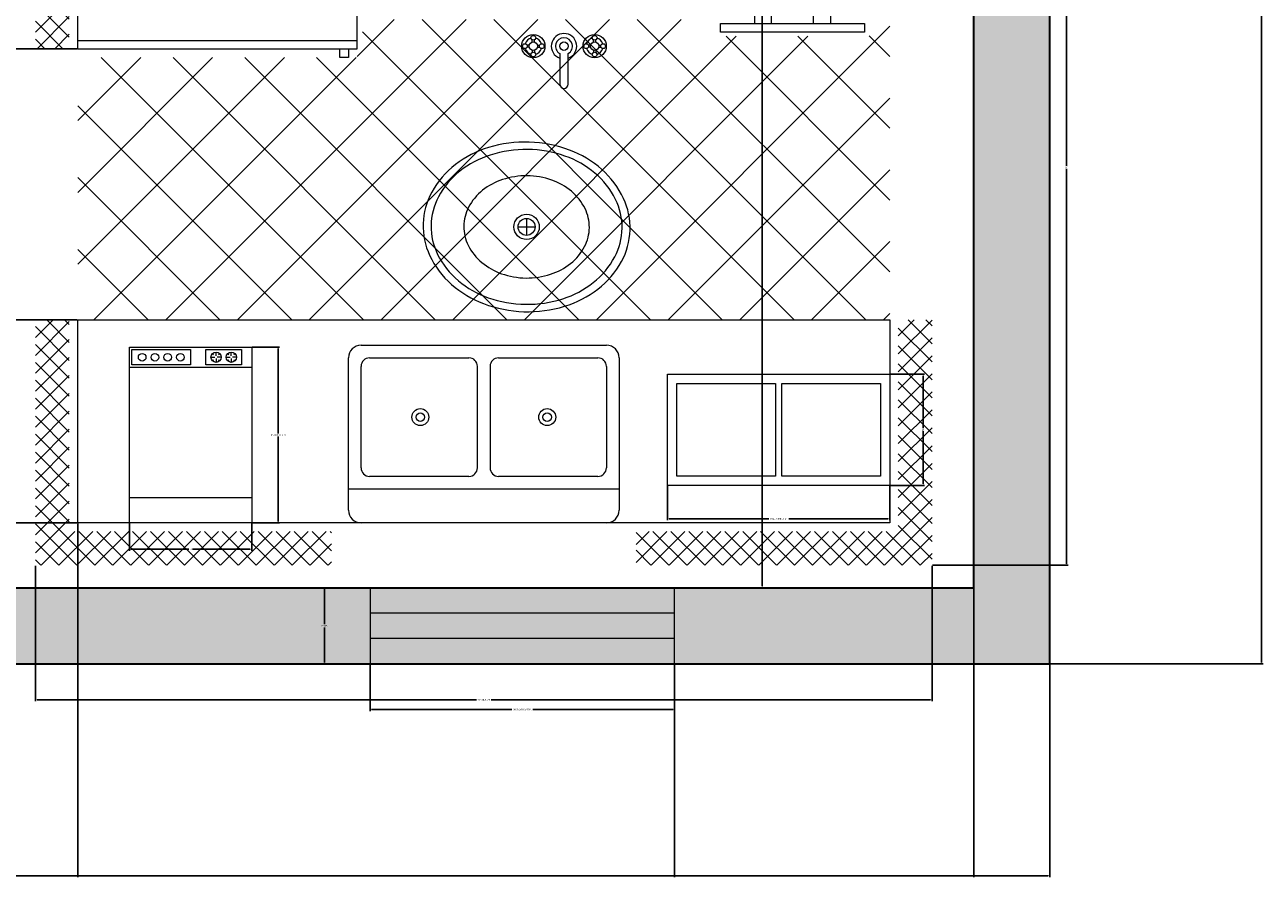
# Model space of a CAD drawing. Units: inches. Extents: x 1434 to 1845, y 1483 to 2014.
# Tile 6 of 11: x 1698 to 1845, y 1483 to 1584. Entities that reach past the tile are written whole.
import ezdxf

# ---------------------------------------------------------------- set-up
doc = ezdxf.new("R2010")
doc.units = ezdxf.units.IN
for name, color, linetype, lineweight in [('A-ANNO-DIMS', 2, 'Continuous', 18), ('A-EQPM', 9, 'Continuous', 18), ('A-FLOR-CASE', 8, 'Continuous', 18), ('A-FLOR-FIXT', 8, 'Continuous', 18), ('A-GLAZ', 4, 'Continuous', 18), ('A-GLAZ-PATT', 9, 'Continuous', 13), ('A-WALL', 7, 'Continuous', 35), ('A-WALL-PATT', 8, 'Continuous', 13)]:
    doc.layers.add(name, color=color, linetype=linetype, lineweight=lineweight)
doc.styles.get("Standard").update_dxf_attribs({"font": 'arial.ttf'})
doc.dimstyles.get("Standard").update_dxf_attribs({"dimtxt": 0.18, "dimasz": 0.18, "dimexe": 0.18, "dimexo": 0.0625, "dimgap": 0.09, "dimtad": 0, "dimtih": 1, "dimtoh": 1, "dimdec": 4, "dimzin": 0, "dimdsep": 46, "dimtxsty": 'Standard', "dimcen": 0.09, "dimadec": 0, "dimazin": 0, "dimtfac": 1, "dimtdec": 4, "dimtofl": 0, "dimtmove": 0, "dimatfit": 3, "dimfxl": 1, "dimtolj": 1, "dimtzin": 0, "dimarcsym": 0})

# ---------------------------------------------------------------- blocks, each defined once
blk = doc.blocks.new('Sink - Oval top')
for p, q in [((-1, 0), (1, 0)), ((0, 1), (0, -1))]:
    blk.add_line(p, q)
for points in [[(-12.23, 0.39, 0.117634), (-11.46, -3.36, 0.104469), (-8.88, -6.8, 0.090016), (-5.08, -9.07, 0.08192), (-0.32, -10.02, 0.08192), (4.49, -9.38, 0.090016), (8.42, -7.36, 0.104469), (11.22, -4.09, 0.117634), (12.23, -0.39, 0.117634), (11.46, 3.36, 0.104469), (8.88, 6.8, 0.090016), (5.08, 9.07, 0.08192), (0.32, 10.02, 0.08192), (-4.49, 9.38, 0.090016), (-8.42, 7.36, 0.104469), (-11.22, 4.09, 0.117634)], [(-11.29, 0.16, 0.118622), (-10.52, -3.25, 0.104678), (-8.07, -6.36, 0.089562), (-4.54, -8.37, 0.081185), (-0.13, -9.15, 0.081185), (4.3, -8.49, 0.089562), (7.89, -6.58, 0.104678), (10.42, -3.55, 0.118622), (11.29, -0.16, 0.118622), (10.52, 3.25, 0.104678), (8.07, 6.36, 0.089562), (4.54, 8.37, 0.081185), (0.13, 9.15, 0.081185), (-4.3, 8.49, 0.089562), (-7.89, 6.58, 0.104678), (-10.42, 3.55, 0.118622)], [(-7.42, 0.08, 0.118283), (-6.91, -2.17, 0.104607), (-5.29, -4.21, 0.089718), (-2.97, -5.53, 0.081436), (-0.07, -6.04, 0.081436), (2.84, -5.59, 0.089718), (5.2, -4.33, 0.104607), (6.86, -2.32, 0.118283), (7.42, -0.08, 0.118283), (6.91, 2.17, 0.104607), (5.29, 4.21, 0.089718), (2.97, 5.53, 0.081436), (0.07, 6.04, 0.081436), (-2.84, 5.59, 0.089718), (-5.2, 4.33, 0.104607), (-6.86, 2.32, 0.118283)]]:
    blk.add_lwpolyline(points, format="xyb", close=True)
for radius in [1.5, 1]:
    blk.add_circle((0, 0), radius)
blk = doc.blocks.new('Faucet - Bathroom top')
for p, q in [((-4.107, 0.125), (-4.375, 0.125)), ((-3.75, 0.4788), (-3.75, 0.75)), ((-3.5, 0.482), (-3.5, 0.75)), ((-3.1461, 0.125), (-2.875, 0.125)), ((3.143, 0.125), (2.875, 0.125)), ((3.5, 0.4788), (3.5, 0.75)), ((3.75, 0.482), (3.75, 0.75)), ((4.1039, 0.125), (4.375, 0.125)), ((-4.1039, -0.125), (-4.375, -0.125)), ((-3.75, -0.4821), (-3.75, -0.75)), ((-3.5, -0.4789), (-3.5, -0.75)), ((-3.143, -0.125), (-2.875, -0.125)), ((-0.5, -0.8639), (-0.5, -4.5)), ((0.5, -4.5), (0.5, -0.8631)), ((3.1461, -0.125), (2.875, -0.125)), ((3.5, -0.4821), (3.5, -0.75)), ((3.75, -0.4789), (3.75, -0.75)), ((4.107, -0.125), (4.375, -0.125))]:
    blk.add_line(p, q)
for centre, radius in [((-3.625, 0), 1.375), ((-4.625, 0), 0.2795), ((-3.625, 0), 0.5), ((-3.625, 1), 0.2795), ((-2.625, 0), 0.2795), ((0, 0), 0.5), ((3.625, 0), 1.375), ((2.625, 0), 0.2795), ((3.625, 0), 0.5), ((3.625, 1), 0.2795), ((4.625, 0), 0.2795), ((-3.625, -1), 0.2795), ((3.625, -1), 0.2795)]:
    blk.add_circle(centre, radius)
for centre, radius, start, end in [((0, 0), 1.5, 289.6514, 250.3603), ((-3.625, 0), 1, 105.2407, 164.2093), ((-3.625, 0), 1, 16.44125, 74.07887), ((0, 0), 1, 300.3431, 239.7554), ((3.625, 0), 1, 106.12, 164.0884), ((3.625, 0), 1, 16.23422, 73.90469), ((-3.625, 0), 1, 196.2342, 253.9047), ((-3.625, 0), 1, 286.12, 344.0884), ((3.625, 0), 1, 196.4413, 254.0789), ((3.625, 0), 1, 285.2407, 344.2093), ((0, -4.5), 0.5, 180, 0)]:
    blk.add_arc(centre, radius, start, end)
blk = doc.blocks.new('Kitchen Layout - 7 x 8 ft')
for p, q in [((-5, 81.32), (2.68, 89)), ((-5, 83.44), (0.56, 89)), ((-5, 85.56), (-1.56, 89)), ((-5, 87.68), (-3.68, 89)), ((-1, 84.97), (-5, 88.97)), ((1.09, 85), (-2.91, 89)), ((3.21, 85), (-0.79, 89)), ((0.81, 85), (4.81, 89)), ((5.34, 85), (1.34, 89)), ((2.93, 85), (6.93, 89)), ((7.46, 85), (3.46, 89)), ((5.05, 85), (9.05, 89)), ((9.58, 85), (5.58, 89)), ((7.17, 85), (11.17, 89)), ((11.7, 85), (7.7, 89)), ((9.29, 85), (13.29, 89)), ((13.82, 85), (9.82, 89)), ((11.41, 85), (15.41, 89)), ((15.94, 85), (11.94, 89)), ((13.53, 85), (17.53, 89)), ((18.06, 85), (14.06, 89)), ((15.65, 85), (19.65, 89)), ((20.18, 85), (16.18, 89)), ((17.78, 85), (21.78, 89)), ((22.31, 85), (18.31, 89)), ((19.9, 85), (23.9, 89)), ((24.43, 85), (20.43, 89)), ((22.02, 85), (26.02, 89)), ((26.55, 85), (22.55, 89)), ((24.14, 85), (28.14, 89)), ((28.67, 85), (24.67, 89)), ((26.26, 85), (30.26, 89)), ((30.79, 85), (26.79, 89)), ((28.38, 85), (32.38, 89)), ((32.91, 85), (28.91, 89)), ((30.5, 85), (34.5, 89)), ((35.03, 85), (31.03, 89)), ((32.63, 85), (36.63, 89)), ((37.16, 85), (33.16, 89)), ((34.75, 85), (38.75, 89)), ((39.28, 85), (35.28, 89)), ((36.87, 85), (40.87, 89)), ((41.4, 85), (37.4, 89)), ((38.99, 85), (42.99, 89)), ((43.52, 85), (39.52, 89)), ((41.11, 85), (45.11, 89)), ((45.64, 85), (41.64, 89)), ((43.23, 85), (47.23, 89)), ((47.76, 85), (43.76, 89)), ((45.35, 85), (49.35, 89)), ((49.88, 85), (45.88, 89)), ((47.47, 85), (51.47, 89)), ((52, 85), (48, 89)), ((49.6, 85), (53.6, 89)), ((54.13, 85), (50.13, 89)), ((51.72, 85), (55.72, 89)), ((56.25, 85), (52.25, 89)), ((53.84, 85), (57.84, 89)), ((58.37, 85), (54.37, 89)), ((55.96, 85), (59.96, 89)), ((60.49, 85), (56.49, 89)), ((58.08, 85), (62.08, 89)), ((62.61, 85), (58.61, 89)), ((60.2, 85), (64.2, 89)), ((64.73, 85), (60.73, 89)), ((62.32, 85), (66.32, 89)), ((66.85, 85), (62.85, 89)), ((64.45, 85), (68.45, 89)), ((68.97, 85), (64.97, 89)), ((66.57, 85), (70.57, 89)), ((71.1, 85), (67.1, 89)), ((68.69, 85), (72.69, 89)), ((73.22, 85), (69.22, 89)), ((70.81, 85), (74.81, 89)), ((75.34, 85), (71.34, 89)), ((72.93, 85), (76.93, 89)), ((77.46, 85), (73.46, 89)), ((75.05, 85), (79.05, 89)), ((79.58, 85), (75.58, 89)), ((77.17, 85), (81.17, 89)), ((81.7, 85), (77.7, 89)), ((79.29, 85), (83.29, 89)), ((83.82, 85), (79.82, 89)), ((81.42, 85), (85.42, 89)), ((85.95, 85), (81.95, 89)), ((83.54, 85), (87.54, 89)), ((88.07, 85), (84.07, 89)), ((85.66, 85), (89.66, 89)), ((90.19, 85), (86.19, 89)), ((87.78, 85), (91.78, 89)), ((92.31, 85), (88.31, 89)), ((89.9, 85), (93.9, 89)), ((94.43, 85), (90.43, 89)), ((92.02, 85), (96.02, 89)), ((96.55, 85), (92.55, 89)), ((94.14, 85), (98.14, 89)), ((101, 82.67), (94.67, 89)), ((96.27, 85), (100.27, 89)), ((101, 84.79), (96.79, 89)), ((101, 86.92), (98.92, 89)), ((-1, 82.85), (-5, 86.85)), ((97, 83.61), (101, 87.61)), ((97, 81.49), (101, 85.49)), ((-1, 80.73), (-5, 84.73)), ((34, 84), (96, 84)), ((34, 60), (34, 84)), ((96, 84), (96, 60)), ((101, 80.55), (97, 84.55)), ((-5, 79.19), (-1, 83.19)), ((-1, 78.61), (-5, 82.61)), ((97, 79.37), (101, 83.37)), ((101, 78.43), (97, 82.43)), ((-5, 77.07), (-1, 81.07)), ((74, 81), (95, 81)), ((97, 77.25), (101, 81.25)), ((-1, 76.49), (-5, 80.49)), ((101, 76.31), (97, 80.31)), ((97, 75.13), (101, 79.13)), ((-5, 74.95), (-1, 78.95)), ((-1, 74.36), (-5, 78.36)), ((101, 74.19), (97, 78.19)), ((-5, 72.83), (-1, 76.83)), ((-1, 72.24), (-5, 76.24)), ((97, 73.01), (101, 77.01)), ((-5, 70.71), (-1, 74.71)), ((101, 72.07), (97, 76.07)), ((97, 70.89), (101, 74.89)), ((-1, 70.12), (-5, 74.12)), ((101, 69.95), (97, 73.95)), ((-5, 68.59), (-1, 72.59)), ((-1, 68), (-5, 72)), ((97, 68.76), (101, 72.76)), ((101, 67.82), (97, 71.82)), ((-5, 66.47), (-1, 70.47)), ((97, 66.64), (101, 70.64)), ((-1, 65.88), (-5, 69.88)), ((101, 65.7), (97, 69.7)), ((-5, 64.35), (-1, 68.35)), ((-1, 63.76), (-5, 67.76)), ((97, 64.52), (101, 68.52)), ((101, 63.58), (97, 67.58)), ((-5, 62.22), (-1, 66.22)), ((97, 62.4), (101, 66.4)), ((-1, 61.64), (-5, 65.64)), ((101, 61.46), (97, 65.46)), ((-5, 60.1), (-1, 64.1)), ((-1, 59.52), (-5, 63.52)), ((97, 60.28), (101, 64.28)), ((100.34, 60), (97, 63.34)), ((-5, 57.98), (-1, 61.98)), ((98.84, 60), (101, 62.16)), ((-1, 57.39), (-5, 61.39)), ((98.22, 60), (97, 61.22)), ((100.96, 60), (101, 60.04)), ((-1.73, 56), (-5, 59.27)), ((-4.86, 56), (-1, 59.86)), ((10.4, 24), (45.9, 59.5)), ((18.88, 24), (54.38, 59.5)), ((27.37, 24), (62.87, 59.5)), ((33.03, 55.11), (37.41, 59.5)), ((96, 60), (34, 60)), ((35.85, 24), (71.35, 59.5)), ((76.2, 24), (40.7, 59.5)), ((84.68, 24), (49.18, 59.5)), ((93.17, 24), (57.67, 59.5)), ((61.31, 24), (96, 58.69)), ((96, 29.65), (66.15, 59.5)), ((80, 60), (80, 59)), ((82, 59), (82, 60)), ((87, 59), (87, 60)), ((89, 60), (89, 59)), ((-3.85, 56), (-5, 57.15)), ((-2.74, 56), (-1, 57.74)), ((67.71, 24), (33.68, 58.04)), ((44.34, 24), (77.84, 57.5)), ((52.82, 24), (86.32, 57.5)), ((96, 38.14), (76.64, 57.5)), ((96, 46.63), (85.13, 57.5)), ((96, 55.11), (93.57, 57.54)), ((0, 57), (33, 57)), ((31, 55), (31, 56)), ((32, 56), (32, 55)), ((0, 30.57), (24.43, 55)), ((0, 39.06), (15.94, 55)), ((0, 47.54), (7.46, 55)), ((1.91, 24), (32.91, 55)), ((33.77, 24), (2.77, 55)), ((42.26, 24), (11.26, 55)), ((50.74, 24), (19.74, 55)), ((59.23, 24), (28.23, 55)), ((32, 55), (31, 55)), ((69.79, 24), (96, 50.21)), ((25.29, 24), (0, 49.29)), ((78.28, 24), (96, 41.72)), ((16.8, 24), (0, 40.8)), ((8.32, 24), (0, 32.32)), ((86.76, 24), (96, 33.24)), ((-5, 21.92), (-2.92, 24)), ((-5, 19.8), (-1, 23.8)), ((-1, 21.33), (-3.67, 24)), ((-1, 23.45), (-1.55, 24)), ((0, 24), (96, 24)), ((0, 0), (0, 24)), ((95.25, 24), (96, 24.75)), ((96, 24), (96, 0)), ((97, 22.1), (98.9, 24)), ((97, 19.97), (101, 23.97)), ((101, 21.16), (98.16, 24)), ((101, 23.28), (100.28, 24)), ((-1, 19.21), (-5, 23.21)), ((101, 19.03), (97, 23.03)), ((-5, 17.68), (-1, 21.68)), ((-1, 17.09), (-5, 21.09)), ((97, 17.85), (101, 21.85)), ((101, 16.91), (97, 20.91)), ((-5, 15.55), (-1, 19.55)), ((97, 15.73), (101, 19.73)), ((-1, 14.97), (-5, 18.97)), ((47.25, 6.5), (47.25, 18.5)), ((48.75, 18.5), (48.75, 6.5)), ((101, 14.79), (97, 18.79)), ((97, 13.61), (101, 17.61)), ((-5, 13.43), (-1, 17.43)), ((-1, 12.85), (-5, 16.85)), ((101, 12.67), (97, 16.67)), ((-5, 11.31), (-1, 15.31)), ((-1, 10.73), (-5, 14.73)), ((97, 11.49), (101, 15.49)), ((-5, 9.19), (-1, 13.19)), ((101, 10.55), (97, 14.55)), ((97, 9.37), (101, 13.37)), ((-1, 8.6), (-5, 12.6)), ((101, 8.43), (97, 12.43)), ((-5, 7.07), (-1, 11.07)), ((-1, 6.48), (-5, 10.48)), ((97, 7.25), (101, 11.25)), ((101, 6.31), (97, 10.31)), ((-5, 4.95), (-1, 8.95)), ((97, 5.12), (101, 9.12)), ((-1, 4.36), (-5, 8.36)), ((101, 4.18), (97, 8.18)), ((-5, 2.83), (-1, 6.83)), ((-1, 2.24), (-5, 6.24)), ((97, 3), (101, 7)), ((101, 2.06), (97, 6.06)), ((-5, 0.71), (-1, 4.71)), ((97, 0.88), (101, 4.88)), ((-1, 0.12), (-5, 4.12)), ((64, 4), (32, 4)), ((101, -0.06), (97, 3.94)), ((-5, -1.42), (-1, 2.58)), ((2, -5), (-5, 2)), ((93.24, -5), (101, 2.76)), ((101, -2.18), (97, 1.82)), ((-5, -3.54), (-1, 0.46)), ((96, 0), (0, 0)), ((95.36, -5), (101, 0.64)), ((-0.12, -5), (-5, -0.12)), ((-4.34, -5), (-0.34, -1)), ((-2.22, -5), (1.78, -1)), ((-0.1, -5), (3.9, -1)), ((4.12, -5), (0.12, -1)), ((2.02, -5), (6.02, -1)), ((6.24, -5), (2.24, -1)), ((4.14, -5), (8.14, -1)), ((8.36, -5), (4.36, -1)), ((6.27, -5), (10.27, -1)), ((10.48, -5), (6.48, -1)), ((8.39, -5), (12.39, -1)), ((12.6, -5), (8.6, -1)), ((10.51, -5), (14.51, -1)), ((14.73, -5), (10.73, -1)), ((12.63, -5), (16.63, -1)), ((16.85, -5), (12.85, -1)), ((14.75, -5), (18.75, -1)), ((18.97, -5), (14.97, -1)), ((16.87, -5), (20.87, -1)), ((21.09, -5), (17.09, -1)), ((18.99, -5), (22.99, -1)), ((23.21, -5), (19.21, -1)), ((21.11, -5), (25.11, -1)), ((25.33, -5), (21.33, -1)), ((23.24, -5), (27.24, -1)), ((27.45, -5), (23.45, -1)), ((25.36, -5), (29.36, -1)), ((29.57, -5), (25.57, -1)), ((30, -3.3), (27.7, -1)), ((30, -1.18), (29.82, -1)), ((66, -2.54), (67.54, -1)), ((66, -4.66), (69.66, -1)), ((69.88, -5), (66, -1.12)), ((67.78, -5), (71.78, -1)), ((72, -5), (68, -1)), ((69.9, -5), (73.9, -1)), ((74.12, -5), (70.12, -1)), ((72.03, -5), (76.03, -1)), ((76.24, -5), (72.24, -1)), ((74.15, -5), (78.15, -1)), ((78.36, -5), (74.36, -1)), ((76.27, -5), (80.27, -1)), ((80.49, -5), (76.49, -1)), ((78.39, -5), (82.39, -1)), ((82.61, -5), (78.61, -1)), ((80.51, -5), (84.51, -1)), ((84.73, -5), (80.73, -1)), ((82.63, -5), (86.63, -1)), ((86.85, -5), (82.85, -1)), ((84.75, -5), (88.75, -1)), ((88.97, -5), (84.97, -1)), ((86.88, -5), (90.88, -1)), ((91.09, -5), (87.09, -1)), ((89, -5), (93, -1)), ((93.21, -5), (89.21, -1)), ((91.12, -5), (95.12, -1)), ((95.34, -5), (91.34, -1)), ((97.46, -5), (93.46, -1)), ((99.58, -5), (95.58, -1)), ((101, -4.3), (97, -0.3)), ((-2.25, -5), (-5, -2.25)), ((27.48, -5), (30, -2.48)), ((97.48, -5), (101, -1.48)), ((-4.37, -5), (-5, -4.37)), ((67.76, -5), (66, -3.24)), ((99.6, -5), (101, -3.6)), ((29.6, -5), (30, -4.6))]:
    blk.add_line(p, q)
for points in [[(0, 56), (0, 84), (33, 84), (33, 56)], [(74, 60), (74, 84), (95, 84), (95, 60)], [(76, 58), (76, 59), (93, 59), (93, 58)]]:
    blk.add_lwpolyline(points, close=True)
for points in [[(33.5, 21), (62.5, 21)], [(32, 1.5), (32, 19.5)], [(34.5, 19.5), (46.25, 19.5)], [(49.75, 19.5), (61.5, 19.5)], [(64, 19.5), (64, 1.5)], [(33.5, 6.5), (33.5, 18.5)], [(62.5, 18.5), (62.5, 6.5)], [(46.25, 5.5), (34.5, 5.5)], [(61.5, 5.5), (49.75, 5.5)], [(62.5, 0), (33.5, 0)]]:
    blk.add_lwpolyline(points)
for centre, radius in [((80, 75), 4), ((80, 75), 3), ((89, 75), 3), ((80, 75), 2), ((89, 75), 2), ((80, 75), 1), ((89, 75), 1), ((80, 66), 3), ((89, 66), 4), ((89, 66), 3), ((80, 66), 2), ((89, 66), 2), ((80, 66), 1), ((89, 66), 1), ((40.5, 12.5), 1), ((55.5, 12.5), 1), ((40.5, 12.5), 0.5), ((55.5, 12.5), 0.5)]:
    blk.add_circle(centre, radius)
for centre, radius, start, end in [((33.5, 19.5), 1.5, 90, 180), ((62.5, 19.5), 1.5, 0, 90), ((34.5, 18.5), 1, 90, 180), ((46.25, 18.5), 1, 0, 90), ((49.75, 18.5), 1, 90, 180), ((61.5, 18.5), 1, 0, 90), ((34.5, 6.5), 1, 180, 270), ((46.25, 6.5), 1, 270, 0), ((49.75, 6.5), 1, 180, 270), ((61.5, 6.5), 1, 270, 0), ((33.5, 1.5), 1.5, 180, 270), ((62.5, 1.5), 1.5, 270, 0)]:
    blk.add_arc(centre, radius, start, end)
blk = doc.blocks.new('Dishwasher')
for p, q in [((16, 32.5), (16.75, 32.5)), ((16.5, 32), (16.2942, 31.7942)), ((16.3156, 33.1843), (16.5, 33)), ((17, 32.75), (17, 33.5)), ((17, 32.25), (17, 31.5)), ((18, 32.5), (17.25, 32.5)), ((17.5, 33), (17.6938, 33.1938)), ((17.7061, 31.7939), (17.5, 32)), ((19, 32.5), (19.75, 32.5)), ((19.5, 32), (19.2942, 31.7942)), ((19.3156, 33.1843), (19.5, 33)), ((20, 32.75), (20, 33.5)), ((20, 32.25), (20, 31.5)), ((21, 32.5), (20.25, 32.5)), ((20.5, 33), (20.6938, 33.1938)), ((20.7061, 31.7939), (20.5, 32)), ((24, 30.5), (0, 30.5)), ((0, 5), (24, 5))]:
    blk.add_line(p, q)
for points in [[(0, 0), (0, 34.5), (24, 34.5), (24, 0)], [(0.5, 31), (0.5, 34), (12, 34), (12, 31)], [(15, 31), (15, 34), (22, 34), (22, 31)]]:
    blk.add_lwpolyline(points, close=True)
for centre, radius in [((2.5, 32.5), 0.75), ((5, 32.5), 0.75), ((7.5, 32.5), 0.75), ((10, 32.5), 0.75), ((17, 32.5), 1), ((20, 32.5), 1)]:
    blk.add_circle(centre, radius)
blk = doc.blocks.new('Wall Cabinet - 18 x 36 in front')
for p, q in [((17.5, -1.5), (17.5, -16.5)), ((18.5, -16.5), (18.5, -1.5))]:
    blk.add_line(p, q)
blk.add_lwpolyline([(0, -18), (0, 0), (36, 0), (36, -18)], close=True)
for points in [[(17.5, -16.5), (1.5, -16.5), (1.5, -1.5), (17.5, -1.5)], [(18.5, -1.5), (34.5, -1.5), (34.5, -16.5), (18.5, -16.5)]]:
    blk.add_lwpolyline(points)
blk = doc.blocks.new('WIN-36IN-9IN')
for p, q in [((3, 36), (3, 0)), ((6, 36), (6, 0))]:
    blk.add_line(p, q)
blk.add_lwpolyline([(9, 0), (9, 36), (0, 36), (0, 0)], close=True)
blk = doc.blocks.new('*D28')
at = {"layer": 'A-ANNO-DIMS', "color": 0, "lineweight": -2, "transparency": 16777216}
for p, q in [((1739.11, 1508.29), (1739.11, 1502.78)), ((1775.11, 1508.29), (1775.11, 1502.78)), ((1739.29, 1502.96), (1755.88, 1502.96)), ((1774.93, 1502.96), (1758.35, 1502.96))]:
    blk.add_line(p, q, dxfattribs=at)
at = {"layer": 'A-ANNO-DIMS', "color": 0, "transparency": 16777216}
for points in [[(1739.29, 1502.99), (1739.29, 1502.93), (1739.11, 1502.96)], [(1774.93, 1502.99), (1774.93, 1502.93), (1775.11, 1502.96)]]:
    blk.add_solid(points, dxfattribs=at)
at = {"layer": 'Defpoints', "color": 0, "transparency": 16777216}
for p in [(1739.11, 1508.36), (1775.11, 1508.36), (1775.11, 1502.96)]:
    blk.add_point(p, dxfattribs=at)
at = {"layer": 'A-ANNO-DIMS', "color": 0, "transparency": 16777216, "insert": (1757.11, 1502.96), "char_height": 0.18, "attachment_point": 5}
blk.add_mtext('\\A1;WINDOW B 36 TYP.', dxfattribs=at)
blk = doc.blocks.new('*D29')
at = {"layer": 'A-ANNO-DIMS', "color": 0, "lineweight": -2, "transparency": 16777216}
for p, q in [((1739.05, 1517.36), (1733.53, 1517.36)), ((1733.71, 1517.18), (1733.71, 1513.04)), ((1733.71, 1508.54), (1733.71, 1512.67)), ((1739.05, 1508.36), (1733.53, 1508.36))]:
    blk.add_line(p, q, dxfattribs=at)
at = {"layer": 'A-ANNO-DIMS', "color": 0, "transparency": 16777216}
for points in [[(1733.68, 1517.18), (1733.74, 1517.18), (1733.71, 1517.36)], [(1733.68, 1508.54), (1733.74, 1508.54), (1733.71, 1508.36)]]:
    blk.add_solid(points, dxfattribs=at)
at = {"layer": 'Defpoints', "color": 0, "transparency": 16777216}
for p in [(1739.11, 1517.36), (1733.71, 1508.36), (1739.11, 1508.36)]:
    blk.add_point(p, dxfattribs=at)
at = {"layer": 'A-ANNO-DIMS', "color": 0, "transparency": 16777216, "insert": (1733.71, 1512.86), "char_height": 0.18, "attachment_point": 5}
blk.add_mtext('\\A1;9 TYP.', dxfattribs=at)
blk = doc.blocks.new('*D46')
at = {"layer": 'A-ANNO-DIMS', "color": 0, "lineweight": -2, "transparency": 16777216}
for p, q in [((1699.55, 1519.96), (1699.55, 1503.94)), ((1805.55, 1519.96), (1805.55, 1503.94)), ((1699.73, 1504.12), (1751.68, 1504.12)), ((1805.37, 1504.12), (1753.42, 1504.12))]:
    blk.add_line(p, q, dxfattribs=at)
at = {"layer": 'A-ANNO-DIMS', "color": 0, "transparency": 16777216}
for points in [[(1699.73, 1504.15), (1699.73, 1504.09), (1699.55, 1504.12)], [(1805.37, 1504.15), (1805.37, 1504.09), (1805.55, 1504.12)]]:
    blk.add_solid(points, dxfattribs=at)
at = {"layer": 'Defpoints', "color": 0, "transparency": 16777216}
for p in [(1699.55, 1520.02), (1805.55, 1520.02), (1805.55, 1504.12)]:
    blk.add_point(p, dxfattribs=at)
at = {"layer": 'A-ANNO-DIMS', "color": 0, "transparency": 16777216, "insert": (1752.55, 1504.12), "char_height": 0.18, "attachment_point": 5}
blk.add_mtext('\\A1;KITCHEN 106', dxfattribs=at)
blk = doc.blocks.new('*D47')
at = {"layer": 'A-ANNO-DIMS', "color": 0, "lineweight": -2, "transparency": 16777216}
for p, q in [((1805.61, 1614.02), (1821.63, 1614.02)), ((1821.45, 1613.84), (1821.45, 1567.2)), ((1821.45, 1520.2), (1821.45, 1566.84)), ((1805.61, 1520.02), (1821.63, 1520.02))]:
    blk.add_line(p, q, dxfattribs=at)
at = {"layer": 'A-ANNO-DIMS', "color": 0, "transparency": 16777216}
for points in [[(1821.42, 1613.84), (1821.48, 1613.84), (1821.45, 1614.02)], [(1821.42, 1520.2), (1821.48, 1520.2), (1821.45, 1520.02)]]:
    blk.add_solid(points, dxfattribs=at)
at = {"layer": 'Defpoints', "color": 0, "transparency": 16777216}
for p in [(1805.55, 1614.02), (1821.45, 1614.02), (1805.55, 1520.02)]:
    blk.add_point(p, dxfattribs=at)
at = {"layer": 'A-ANNO-DIMS', "color": 0, "transparency": 16777216, "insert": (1821.45, 1567.02), "char_height": 0.18, "attachment_point": 5}
blk.add_mtext('\\A1;94', dxfattribs=at)
blk = doc.blocks.new('*D50')
at = {"layer": 'A-ANNO-DIMS', "color": 0, "lineweight": -2, "transparency": 16777216}
for p, q in [((1725.18, 1545.8), (1728.41, 1545.8)), ((1728.23, 1545.62), (1728.23, 1535.59)), ((1728.23, 1525.2), (1728.23, 1535.23)), ((1725.18, 1525.02), (1728.41, 1525.02))]:
    blk.add_line(p, q, dxfattribs=at)
at = {"layer": 'A-ANNO-DIMS', "color": 0, "transparency": 16777216}
for points in [[(1728.2, 1545.62), (1728.26, 1545.62), (1728.23, 1545.8)], [(1728.2, 1525.2), (1728.26, 1525.2), (1728.23, 1525.02)]]:
    blk.add_solid(points, dxfattribs=at)
at = {"layer": 'Defpoints', "color": 0, "transparency": 16777216}
for p in [(1725.11, 1545.8), (1728.23, 1545.8), (1725.11, 1525.02)]:
    blk.add_point(p, dxfattribs=at)
at = {"layer": 'A-ANNO-DIMS', "color": 0, "transparency": 16777216, "insert": (1728.23, 1535.41), "char_height": 0.18, "attachment_point": 5}
blk.add_mtext('\\A1;DISHWASHER 21', dxfattribs=at)
blk = doc.blocks.new('*D51')
at = {"layer": 'A-ANNO-DIMS', "color": 0, "lineweight": -2, "transparency": 16777216}
for p, q in [((1710.66, 1524.96), (1710.66, 1521.72)), ((1725.11, 1524.96), (1725.11, 1521.72)), ((1710.84, 1521.9), (1717.68, 1521.9)), ((1724.93, 1521.9), (1718.1, 1521.9))]:
    blk.add_line(p, q, dxfattribs=at)
at = {"layer": 'A-ANNO-DIMS', "color": 0, "transparency": 16777216}
for points in [[(1710.84, 1521.93), (1710.84, 1521.87), (1710.66, 1521.9)], [(1724.93, 1521.93), (1724.93, 1521.87), (1725.11, 1521.9)]]:
    blk.add_solid(points, dxfattribs=at)
at = {"layer": 'Defpoints', "color": 0, "transparency": 16777216}
for p in [(1710.66, 1525.02), (1725.11, 1525.02), (1725.11, 1521.9)]:
    blk.add_point(p, dxfattribs=at)
at = {"layer": 'A-ANNO-DIMS', "color": 0, "transparency": 16777216, "insert": (1717.89, 1521.9), "char_height": 0.18, "attachment_point": 5}
blk.add_mtext('\\A1;14', dxfattribs=at)
blk = doc.blocks.new('*D52')
at = {"layer": 'A-ANNO-DIMS', "color": 0, "lineweight": -2, "transparency": 16777216}
for p, q in [((1774.28, 1529.39), (1774.28, 1525.33)), ((1800.55, 1529.39), (1800.55, 1525.33)), ((1774.46, 1525.51), (1786.24, 1525.51)), ((1800.37, 1525.51), (1788.6, 1525.51))]:
    blk.add_line(p, q, dxfattribs=at)
at = {"layer": 'A-ANNO-DIMS', "color": 0, "transparency": 16777216}
for points in [[(1774.46, 1525.54), (1774.46, 1525.48), (1774.28, 1525.51)], [(1800.37, 1525.54), (1800.37, 1525.48), (1800.55, 1525.51)]]:
    blk.add_solid(points, dxfattribs=at)
at = {"layer": 'Defpoints', "color": 0, "transparency": 16777216}
for p in [(1774.28, 1529.45), (1800.55, 1529.45), (1800.55, 1525.51)]:
    blk.add_point(p, dxfattribs=at)
at = {"layer": 'A-ANNO-DIMS', "color": 0, "transparency": 16777216, "insert": (1787.42, 1525.51), "char_height": 0.18, "attachment_point": 5}
blk.add_mtext('\\A1;WALL CABINET 26', dxfattribs=at)
blk = doc.blocks.new('*D53')
at = {"layer": 'A-ANNO-DIMS', "color": 0, "lineweight": -2, "transparency": 16777216}
for p, q in [((1800.61, 1542.59), (1804.67, 1542.59)), ((1804.49, 1542.41), (1804.49, 1536.2)), ((1804.49, 1529.63), (1804.49, 1535.84)), ((1800.61, 1529.45), (1804.67, 1529.45))]:
    blk.add_line(p, q, dxfattribs=at)
at = {"layer": 'A-ANNO-DIMS', "color": 0, "transparency": 16777216}
for points in [[(1804.46, 1542.41), (1804.52, 1542.41), (1804.49, 1542.59)], [(1804.46, 1529.63), (1804.52, 1529.63), (1804.49, 1529.45)]]:
    blk.add_solid(points, dxfattribs=at)
at = {"layer": 'Defpoints', "color": 0, "transparency": 16777216}
for p in [(1800.55, 1542.59), (1804.49, 1542.59), (1800.55, 1529.45)]:
    blk.add_point(p, dxfattribs=at)
at = {"layer": 'A-ANNO-DIMS', "color": 0, "transparency": 16777216, "insert": (1804.49, 1536.02), "char_height": 0.18, "attachment_point": 5}
blk.add_mtext('\\A1;13', dxfattribs=at)
blk = doc.blocks.new('*D54')
at = {"layer": 'A-ANNO-DIMS', "color": 0, "lineweight": -2, "transparency": 16777216}
for p, q in [((1459.47, 1508.29), (1459.47, 1483.15)), ((1819.47, 1508.29), (1819.47, 1483.15)), ((1459.65, 1483.33), (1639.19, 1483.33)), ((1819.29, 1483.33), (1639.76, 1483.33))]:
    blk.add_line(p, q, dxfattribs=at)
at = {"layer": 'A-ANNO-DIMS', "color": 0, "transparency": 16777216}
for points in [[(1459.65, 1483.36), (1459.65, 1483.3), (1459.47, 1483.33)], [(1819.29, 1483.36), (1819.29, 1483.3), (1819.47, 1483.33)]]:
    blk.add_solid(points, dxfattribs=at)
at = {"layer": 'Defpoints', "color": 0, "transparency": 16777216}
for p in [(1459.47, 1508.36), (1819.47, 1508.36), (1819.47, 1483.33)]:
    blk.add_point(p, dxfattribs=at)
at = {"layer": 'A-ANNO-DIMS', "color": 0, "transparency": 16777216, "insert": (1639.47, 1483.33), "char_height": 0.18, "attachment_point": 5}
blk.add_mtext('\\A1;360', dxfattribs=at)
blk = doc.blocks.new('*D55')
at = {"layer": 'A-ANNO-DIMS', "color": 0, "lineweight": -2, "transparency": 16777216}
for p, q in [((1819.54, 1988.36), (1844.68, 1988.36)), ((1844.5, 1988.18), (1844.5, 1748.54)), ((1844.5, 1508.54), (1844.5, 1748.17)), ((1819.54, 1508.36), (1844.68, 1508.36))]:
    blk.add_line(p, q, dxfattribs=at)
at = {"layer": 'A-ANNO-DIMS', "color": 0, "transparency": 16777216}
for points in [[(1844.47, 1988.18), (1844.53, 1988.18), (1844.5, 1988.36)], [(1844.47, 1508.54), (1844.53, 1508.54), (1844.5, 1508.36)]]:
    blk.add_solid(points, dxfattribs=at)
at = {"layer": 'Defpoints', "color": 0, "transparency": 16777216}
for p in [(1819.47, 1988.36), (1844.5, 1988.36), (1819.47, 1508.36)]:
    blk.add_point(p, dxfattribs=at)
at = {"layer": 'A-ANNO-DIMS', "color": 0, "transparency": 16777216, "insert": (1844.5, 1748.36), "char_height": 0.18, "attachment_point": 5}
blk.add_mtext('\\A1;480', dxfattribs=at)
blk = doc.blocks.new('*D58')
at = {"layer": 'A-ANNO-DIMS', "color": 0, "lineweight": -2, "transparency": 16777216}
for p, q in [((1670.97, 1974.79), (1670.97, 1483.15)), ((1810.47, 1974.79), (1810.47, 1483.15)), ((1671.15, 1483.33), (1740.34, 1483.33)), ((1810.29, 1483.33), (1741.11, 1483.33))]:
    blk.add_line(p, q, dxfattribs=at)
at = {"layer": 'A-ANNO-DIMS', "color": 0, "transparency": 16777216}
for points in [[(1671.15, 1483.36), (1671.15, 1483.3), (1670.97, 1483.33)], [(1810.29, 1483.36), (1810.29, 1483.3), (1810.47, 1483.33)]]:
    blk.add_solid(points, dxfattribs=at)
at = {"layer": 'Defpoints', "color": 0, "transparency": 16777216}
for p in [(1670.97, 1974.86), (1810.47, 1974.86), (1810.47, 1483.33)]:
    blk.add_point(p, dxfattribs=at)
at = {"layer": 'A-ANNO-DIMS', "color": 0, "transparency": 16777216, "insert": (1740.72, 1483.33), "char_height": 0.18, "attachment_point": 5}
blk.add_mtext('\\A1;139.5', dxfattribs=at)
blk = doc.blocks.new('*D67')
at = {"layer": 'A-ANNO-DIMS', "color": 0, "lineweight": -2, "transparency": 16777216}
for p, q in [((1694.97, 1517.42), (1694.97, 2013.56)), ((1695.15, 2013.38), (1752.34, 2013.38)), ((1810.29, 2013.38), (1753.11, 2013.38)), ((1810.47, 1517.42), (1810.47, 2013.56))]:
    blk.add_line(p, q, dxfattribs=at)
at = {"layer": 'A-ANNO-DIMS', "color": 0, "transparency": 16777216}
for points in [[(1695.15, 2013.41), (1695.15, 2013.35), (1694.97, 2013.38)], [(1810.29, 2013.41), (1810.29, 2013.35), (1810.47, 2013.38)]]:
    blk.add_solid(points, dxfattribs=at)
at = {"layer": 'Defpoints', "color": 0, "transparency": 16777216}
for p in [(1810.47, 2013.38), (1694.97, 1517.36), (1810.47, 1517.36)]:
    blk.add_point(p, dxfattribs=at)
at = {"layer": 'A-ANNO-DIMS', "color": 0, "transparency": 16777216, "insert": (1752.72, 2013.38), "char_height": 0.18, "attachment_point": 5}
blk.add_mtext('\\A1;115.5', dxfattribs=at)
blk = doc.blocks.new('*D80')
at = {"layer": 'A-ANNO-DIMS', "color": 0, "lineweight": -2, "transparency": 16777216}
for p, q in [((1775.11, 1508.29), (1775.11, 1483.15)), ((1819.47, 1508.29), (1819.47, 1483.15)), ((1775.29, 1483.33), (1796.9, 1483.33)), ((1819.29, 1483.33), (1797.69, 1483.33))]:
    blk.add_line(p, q, dxfattribs=at)
at = {"layer": 'A-ANNO-DIMS', "color": 0, "transparency": 16777216}
for points in [[(1775.29, 1483.36), (1775.29, 1483.3), (1775.11, 1483.33)], [(1819.29, 1483.36), (1819.29, 1483.3), (1819.47, 1483.33)]]:
    blk.add_solid(points, dxfattribs=at)
at = {"layer": 'Defpoints', "color": 0, "transparency": 16777216}
for p in [(1775.11, 1508.36), (1819.47, 1508.36), (1819.47, 1483.33)]:
    blk.add_point(p, dxfattribs=at)
at = {"layer": 'A-ANNO-DIMS', "color": 0, "transparency": 16777216, "insert": (1797.29, 1483.33), "char_height": 0.18, "attachment_point": 5}
blk.add_mtext('\\A1;44.36', dxfattribs=at)
blk = doc.blocks.new('*D82')
at = {"layer": 'A-ANNO-DIMS', "color": 0, "lineweight": -2, "transparency": 16777216}
for p, q in [((1704.55, 1524.96), (1704.55, 1483.15)), ((1694.97, 1517.29), (1694.97, 1483.15)), ((1695.15, 1483.33), (1699.37, 1483.33)), ((1704.37, 1483.33), (1700.16, 1483.33))]:
    blk.add_line(p, q, dxfattribs=at)
at = {"layer": 'A-ANNO-DIMS', "color": 0, "transparency": 16777216}
for points in [[(1695.15, 1483.36), (1695.15, 1483.3), (1694.97, 1483.33)], [(1704.37, 1483.36), (1704.37, 1483.3), (1704.55, 1483.33)]]:
    blk.add_solid(points, dxfattribs=at)
at = {"layer": 'Defpoints', "color": 0, "transparency": 16777216}
for p in [(1704.55, 1525.02), (1694.97, 1517.36), (1704.55, 1483.33)]:
    blk.add_point(p, dxfattribs=at)
at = {"layer": 'A-ANNO-DIMS', "color": 0, "transparency": 16777216, "insert": (1699.76, 1483.33), "char_height": 0.18, "attachment_point": 5}
blk.add_mtext('\\A1;9.576', dxfattribs=at)
blk = doc.blocks.new('*D83')
at = {"layer": 'A-ANNO-DIMS', "color": 0, "lineweight": -2, "transparency": 16777216}
for p, q in [((1704.49, 1525.02), (1434.27, 1525.02)), ((1434.45, 1524.84), (1434.45, 1521.37)), ((1434.45, 1517.54), (1434.45, 1521.01)), ((1694.91, 1517.36), (1434.27, 1517.36))]:
    blk.add_line(p, q, dxfattribs=at)
at = {"layer": 'A-ANNO-DIMS', "color": 0, "transparency": 16777216}
for points in [[(1434.42, 1524.84), (1434.48, 1524.84), (1434.45, 1525.02)], [(1434.42, 1517.54), (1434.48, 1517.54), (1434.45, 1517.36)]]:
    blk.add_solid(points, dxfattribs=at)
at = {"layer": 'Defpoints', "color": 0, "transparency": 16777216}
for p in [(1704.55, 1525.02), (1434.45, 1517.36), (1694.97, 1517.36)]:
    blk.add_point(p, dxfattribs=at)
at = {"layer": 'A-ANNO-DIMS', "color": 0, "transparency": 16777216, "insert": (1434.45, 1521.19), "char_height": 0.18, "attachment_point": 5}
blk.add_mtext('\\A1;7.664', dxfattribs=at)
blk = doc.blocks.new('*D84')
at = {"layer": 'A-ANNO-DIMS', "color": 0, "lineweight": -2, "transparency": 16777216}
for p, q in [((1704.49, 1581.02), (1434.27, 1581.02)), ((1434.45, 1580.84), (1434.45, 1565.2)), ((1434.45, 1549.2), (1434.45, 1564.84)), ((1704.49, 1549.02), (1434.27, 1549.02))]:
    blk.add_line(p, q, dxfattribs=at)
at = {"layer": 'A-ANNO-DIMS', "color": 0, "transparency": 16777216}
for points in [[(1434.42, 1580.84), (1434.48, 1580.84), (1434.45, 1581.02)], [(1434.42, 1549.2), (1434.48, 1549.2), (1434.45, 1549.02)]]:
    blk.add_solid(points, dxfattribs=at)
at = {"layer": 'Defpoints', "color": 0, "transparency": 16777216}
for p in [(1434.45, 1581.02), (1704.55, 1581.02), (1704.55, 1549.02)]:
    blk.add_point(p, dxfattribs=at)
at = {"layer": 'A-ANNO-DIMS', "color": 0, "transparency": 16777216, "insert": (1434.45, 1565.02), "char_height": 0.18, "attachment_point": 5}
blk.add_mtext('\\A1;32', dxfattribs=at)
blk = doc.blocks.new('*D85')
at = {"layer": 'A-ANNO-DIMS', "color": 0, "lineweight": -2, "transparency": 16777216}
for p, q in [((1810.41, 1675.08), (1785.27, 1675.08)), ((1785.45, 1674.9), (1785.45, 1596.4)), ((1785.45, 1517.54), (1785.45, 1596.04)), ((1810.41, 1517.36), (1785.27, 1517.36))]:
    blk.add_line(p, q, dxfattribs=at)
at = {"layer": 'A-ANNO-DIMS', "color": 0, "transparency": 16777216}
for points in [[(1785.42, 1674.9), (1785.48, 1674.9), (1785.45, 1675.08)], [(1785.42, 1517.54), (1785.48, 1517.54), (1785.45, 1517.36)]]:
    blk.add_solid(points, dxfattribs=at)
at = {"layer": 'Defpoints', "color": 0, "transparency": 16777216}
for p in [(1785.45, 1675.08), (1810.47, 1675.08), (1810.47, 1517.36)]:
    blk.add_point(p, dxfattribs=at)
at = {"layer": 'A-ANNO-DIMS', "color": 0, "transparency": 16777216, "insert": (1785.45, 1596.22), "char_height": 0.18, "attachment_point": 5}
blk.add_mtext('\\A1;157.73', dxfattribs=at)

msp = doc.modelspace()

# ---------------------------------------------------------------- hatches: boundary and pattern name
at = {"layer": 'A-GLAZ-PATT'}
h = msp.add_hatch(color=256, dxfattribs=at)
h.dxf.hatch_style = 1
h.set_gradient(color1=(0, 0, 255), color2=(255, 255, 0), name='INVHEMISPHERICAL')
h.paths.add_polyline_path([(1775.1129, 1517.3553), (1739.1129, 1517.3553), (1739.1129, 1514.3553), (1775.1129, 1514.3553)])
h.paths.add_polyline_path([(1775.1129, 1514.3553), (1739.1129, 1514.3553), (1739.1129, 1511.3553), (1775.1129, 1511.3553)])
h.paths.add_polyline_path([(1775.1129, 1511.3553), (1739.1129, 1511.3553), (1739.1129, 1508.3553), (1775.1129, 1508.3553)])
at = {"layer": 'A-WALL-PATT'}
h = msp.add_hatch(color=256, dxfattribs=at)
h.dxf.hatch_style = 1
h.paths.add_polyline_path([(1472.9742, 1730.3553), (1577.9742, 1730.3553), (1577.9742, 1734.8553), (1573.4742, 1734.8553), (1573.4742, 1815.8553), (1568.9742, 1815.8553), (1568.9742, 1734.8553), (1472.9742, 1734.8553), (1472.9742, 1770.1951), (1459.9742, 1770.1951), (1459.9742, 1782.1951), (1459.9742, 1818.1951), (1472.9742, 1818.1951), (1472.9742, 1854.8553), (1568.9742, 1854.8553), (1568.9742, 1851.8553), (1573.4742, 1851.8553), (1573.4742, 1854.8553), (1573.4742, 1859.3553), (1472.9742, 1859.3553), (1472.9742, 1899.9369), (1459.9742, 1899.9369), (1459.9742, 1911.9369), (1459.9742, 1947.9369), (1472.9742, 1947.9369), (1472.9742, 1974.8553), (1513.9785, 1974.8553), (1513.9785, 1987.8553), (1561.9785, 1987.8553), (1561.9785, 1974.8553), (1612.4742, 1974.8553), (1612.4742, 1859.3553), (1609.4742, 1859.3553), (1609.4742, 1854.8553), (1616.9742, 1854.8553), (1616.9742, 1910.3553), (1625.153, 1910.3553), (1625.153, 1914.8553), (1616.9742, 1914.8553), (1616.9742, 1988.3553), (1459.4742, 1988.3553), (1459.4742, 1508.3553), (1630.4742, 1508.3553), (1630.4742, 1517.3553), (1472.9742, 1517.3553), (1472.9742, 1586.3553), (1616.9742, 1586.3553), (1616.9742, 1583.3553), (1621.4742, 1583.3553), (1621.4742, 1586.3553), (1621.4742, 1734.8553), (1616.9742, 1734.8553), (1613.9742, 1734.8553), (1613.9742, 1730.3553), (1616.9742, 1730.3553), (1616.9742, 1590.8553), (1472.9742, 1590.8553), (1472.9742, 1635.7299), (1459.9742, 1635.7299), (1459.9742, 1647.7299), (1459.9742, 1683.7299), (1472.9742, 1683.7299)])
h.paths.add_polyline_path([(1819.4742, 1773.1667), (1810.4742, 1773.1667), (1810.4742, 1734.8553), (1714.4742, 1734.8553), (1714.4742, 1815.8553), (1709.9742, 1815.8553), (1709.9742, 1730.3553), (1745.9742, 1730.3553), (1745.9742, 1675.0848), (1753.4742, 1675.0848), (1753.4742, 1679.5848), (1750.4742, 1679.5848), (1750.4742, 1730.3553), (1810.4742, 1730.3553), (1810.4742, 1679.5848), (1792.4742, 1679.5848), (1792.4742, 1675.0848), (1810.4742, 1675.0848), (1810.4742, 1517.3553), (1775.1129, 1517.3553), (1775.1129, 1508.3553), (1819.4742, 1508.3553)])
h.paths.add_polyline_path([(1739.1129, 1517.3553), (1694.9742, 1517.3553), (1694.9742, 1730.3553), (1690.4742, 1730.3553), (1690.4742, 1517.3553), (1678.4742, 1517.3553), (1675.4742, 1517.3553), (1672.8212, 1517.3553), (1672.8212, 1508.3553), (1678.4742, 1508.3553), (1739.1129, 1508.3553)])
h.paths.add_polyline_path([(1735.6549, 1987.8553), (1783.6549, 1987.8553), (1783.6549, 1974.8553), (1810.4742, 1974.8553), (1810.4742, 1859.3553), (1709.9742, 1859.3553), (1709.9742, 1854.8553), (1709.9742, 1851.8553), (1714.4742, 1851.8553), (1714.4742, 1854.8553), (1810.4742, 1854.8553), (1810.4742, 1809.1667), (1819.4742, 1809.1667), (1819.4742, 1988.3553), (1666.4742, 1988.3553), (1666.4742, 1914.8553), (1661.1087, 1914.8553), (1661.1087, 1910.3553), (1666.4742, 1910.3553), (1666.4742, 1854.8553), (1673.9742, 1854.8553), (1673.9742, 1859.3553), (1670.9742, 1859.3553), (1670.9742, 1974.8553), (1735.6549, 1974.8553)])

# ---------------------------------------------------------------- linework, layer by layer
at = {"layer": 'A-WALL'}
for p, q in [((1810.4742, 1517.3553), (1810.4742, 1675.0848)), ((1694.9742, 1517.3553), (1810.4742, 1517.3553))]:
    msp.add_line(p, q, dxfattribs=at)
msp.add_lwpolyline([(1678.4742, 1508.3553), (1819.4742, 1508.3553), (1819.4742, 1988.3553), (1459.4742, 1988.3553), (1459.4742, 1508.3553), (1630.4742, 1508.3553)], dxfattribs=at)

# ---------------------------------------------------------------- block references
at = {"layer": 'A-EQPM', "xscale": 0.6022922010833404, "yscale": 0.6022922010833404, "zscale": 0.6022922010833404}
msp.add_blockref('Dishwasher', (1710.6585, 1525.0191), dxfattribs=at)
at = {"layer": 'A-FLOR-CASE', "xscale": 0.7296805008721118, "yscale": 0.7296805008721118, "zscale": 0.7296805008721118}
msp.add_blockref('Wall Cabinet - 18 x 36 in front', (1774.282, 1542.5866), dxfattribs=at)
at = {"layer": 'A-FLOR-FIXT'}
for name, p in [('Kitchen Layout - 7 x 8 ft', (1704.5505, 1525.0191)), ('Faucet - Bathroom top', (1762.0353, 1581.3537)), ('Sink - Oval top', (1757.6134, 1559.9981))]:
    msp.add_blockref(name, p, dxfattribs=at)
at = {"layer": 'A-GLAZ', "rotation": 270.0000000000006}
msp.add_blockref('WIN-36IN-9IN', (1739.1129, 1517.3553), dxfattribs=at)

# ---------------------------------------------------------------- dimensions: what is measured, and where the dimension line sits
at = {"layer": 'A-ANNO-DIMS'}
for base, p1, p2, override, picture, middle in [((1810.4742, 2013.3803), (1694.9742, 1517.3553), (1810.4742, 1517.3553), {"dimdec": 1, "dimlfac": 1, "dimrnd": 0, "dimzin": 0, "dimdsep": 46, "dimlunit": 2}, '*D67', (1752.7242, 2013.3803)), ((1810.4742, 1483.3303), (1670.9742, 1974.8553), (1810.4742, 1974.8553), {"dimdec": 1, "dimlfac": 1, "dimrnd": 0, "dimzin": 0, "dimdsep": 46, "dimlunit": 2}, '*D58', (1740.7242, 1483.3303)), ((1704.5505, 1483.3303), (1694.9742, 1517.3553), (1704.5505, 1525.0191), {"dimdec": 3, "dimlfac": 1, "dimrnd": 0, "dimzin": 0, "dimdsep": 46, "dimlunit": 2}, '*D82', (1699.7623, 1483.3303)), ((1725.1135, 1521.9022), (1710.6585, 1525.0191), (1725.1135, 1525.0191), {"dimdec": 0, "dimlfac": 1, "dimrnd": 0, "dimzin": 0, "dimdsep": 46, "dimlunit": 2}, '*D51', (1717.886, 1521.9022)), ((1819.4742, 1483.3303), (1459.4742, 1508.3553), (1819.4742, 1508.3553), {"dimdec": 0, "dimlfac": 1, "dimrnd": 0, "dimzin": 0, "dimdsep": 46, "dimlunit": 2}, '*D54', (1639.4742, 1483.3303)), ((1819.4742, 1483.3303), (1775.1129, 1508.3553), (1819.4742, 1508.3553), {"dimdec": 2, "dimlfac": 1, "dimrnd": 0, "dimzin": 0, "dimdsep": 46, "dimlunit": 2}, '*D80', (1797.2936, 1483.3303))]:
    dim = msp.add_linear_dim(base=base, p1=p1, p2=p2, dimstyle='Standard', override=override, dxfattribs=at)
    dim.commit()
    dim.dimension.update_dxf_attribs({"geometry": picture, "text_midpoint": middle})
for base, p1, p2, override, picture, middle in [((1844.4992, 1988.3553), (1819.4742, 1508.3553), (1819.4742, 1988.3553), {"dimdec": 0, "dimlfac": 1, "dimrnd": 0, "dimzin": 0, "dimdsep": 46, "dimlunit": 2}, '*D55', (1844.4992, 1748.3553)), ((1785.4492, 1675.0848), (1810.4742, 1517.3553), (1810.4742, 1675.0848), {"dimdec": 2, "dimlfac": 1, "dimrnd": 0, "dimzin": 0, "dimdsep": 46, "dimlunit": 2}, '*D85', (1785.4492, 1596.2201)), ((1821.4505, 1614.0191), (1805.5505, 1520.0191), (1805.5505, 1614.0191), {"dimdec": 0, "dimlfac": 1, "dimrnd": 0, "dimzin": 0, "dimdsep": 46, "dimlunit": 2}, '*D47', (1821.4505, 1567.0191)), ((1434.4492, 1581.019), (1704.5505, 1549.0191), (1704.5505, 1581.019), {"dimdec": 0, "dimlfac": 1, "dimrnd": 0, "dimzin": 0, "dimdsep": 46, "dimlunit": 2}, '*D84', (1434.4492, 1565.0191)), ((1804.4907, 1542.5866), (1800.5505, 1529.4523), (1800.5505, 1542.5866), {"dimdec": 0, "dimlfac": 1, "dimrnd": 0, "dimzin": 0, "dimdsep": 46, "dimlunit": 2}, '*D53', (1804.4907, 1536.0194)), ((1434.4492, 1517.3553), (1704.5505, 1525.0191), (1694.9742, 1517.3553), {"dimdec": 3, "dimlfac": 1, "dimrnd": 0, "dimzin": 0, "dimdsep": 46, "dimlunit": 2}, '*D83', (1434.4492, 1521.1872))]:
    dim = msp.add_linear_dim(base=base, p1=p1, p2=p2, angle=90, dimstyle='Standard', override=override, dxfattribs=at)
    dim.commit()
    dim.dimension.update_dxf_attribs({"geometry": picture, "text_midpoint": middle})
for base, p1, p2, angle, text, picture, middle in [((1728.2304, 1545.7982), (1725.1135, 1525.0191), (1725.1135, 1545.7982), 90, 'DISHWASHER <>', '*D50', (1728.2304, 1535.4086)), ((1733.7129, 1508.3553), (1739.1129, 1517.3553), (1739.1129, 1508.3553), 270, '<> TYP.', '*D29', (1733.7129, 1512.8553)), ((1775.1129, 1502.9553), (1739.1129, 1508.3553), (1775.1129, 1508.3553), 0, 'WINDOW B <> TYP.', '*D28', (1757.1129, 1502.9553))]:
    dim = msp.add_linear_dim(base=base, p1=p1, p2=p2, angle=angle, text=text, dimstyle='Standard', override={"dimdec": 0, "dimlfac": 1, "dimrnd": 0, "dimzin": 0, "dimdsep": 46, "dimlunit": 2}, dxfattribs=at)
    dim.commit()
    dim.dimension.update_dxf_attribs({"geometry": picture, "text_midpoint": middle})
for base, p1, p2, text, picture, middle in [((1800.5505, 1525.512), (1774.282, 1529.4523), (1800.5505, 1529.4523), 'WALL CABINET <>', '*D52', (1787.4162, 1525.512)), ((1805.5505, 1504.1191), (1699.5505, 1520.0191), (1805.5505, 1520.0191), 'KITCHEN <>', '*D46', (1752.5505, 1504.1191))]:
    dim = msp.add_linear_dim(base=base, p1=p1, p2=p2, text=text, dimstyle='Standard', override={"dimdec": 0, "dimlfac": 1, "dimrnd": 0, "dimzin": 0, "dimdsep": 46, "dimlunit": 2}, dxfattribs=at)
    dim.commit()
    dim.dimension.update_dxf_attribs({"geometry": picture, "text_midpoint": middle})

doc.saveas('drawing.dxf')
